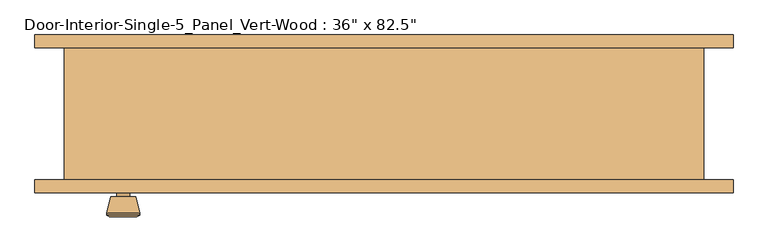
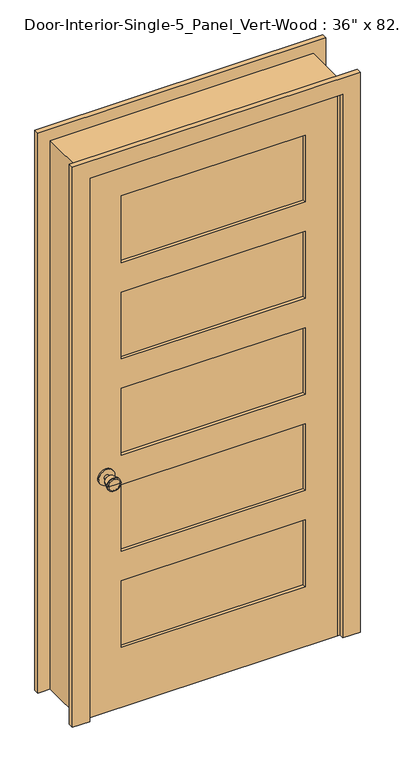
"""IFC4 building model written with IfcOpenShell, lengths in millimetres: door geometry."""

from ifc_helpers import new_model, si_unit, point, frame, frame_2d, origin, place, context, project, spatial, polyline, circle_curve, trimmed, segment, composite_curve, outline, extrude, faceted_brep, source, transform, mapped, element, save
from ifc_brep_helpers import plane_surface, cylinder_surface, revolved_surface, advanced_brep


def door_bc447172(model_context):
    return source(origin(), model_context, "Body", "SolidModel", [
        advanced_brep(
        [(-393.7, -55.9, 914.4), (-403.7, -55.9, 914.4), (-383.7, -55.9, 914.4), (-373.2241324, -6.9, 914.4), (-414.1758676, -6.9, 914.4), (-393.7, -6.9, 914.4), (-368.7, -8.7278681, 914.4), (-418.7, -8.7278681, 914.4), (-368.7, -12.1915463, 914.4), (-418.7, -12.1915463, 914.4), (-375.063764, -36.9, 914.4), (-412.336236, -36.9, 914.4), (-383.7, -36.9, 914.4), (-403.7, -36.9, 914.4)],
        [
            (0, 1),
            (1, 2, circle_curve(frame((-393.7, -55.9, 914.4), z_axis=(0.0, -1.0, 0.0), x_axis=(-1.0, 0.0, 0.0)), 10.0)),
            (2, 0),
            (2, 1, circle_curve(frame((-393.7, -55.9, 914.4), z_axis=(0.0, -1.0, 0.0), x_axis=(-1.0, 0.0, 0.0)), 10.0)),
            (3, 4, circle_curve(frame((-393.7, -6.9, 914.4), z_axis=(0.0, 1.0, 0.0), x_axis=(-1.0, 0.0, 0.0)), 20.4758676)),
            (4, 5),
            (5, 3),
            (4, 3, circle_curve(frame((-393.7, -6.9, 914.4), z_axis=(0.0, 1.0, 0.0), x_axis=(-1.0, 0.0, 0.0)), 20.4758676)),
            (6, 7, circle_curve(frame((-393.7, -8.7278681, 914.4), z_axis=(0.0, 1.0, 0.0), x_axis=(-1.0, 0.0, 0.0)), 25.0)),
            (7, 4),
            (3, 6),
            (7, 6, circle_curve(frame((-393.7, -8.7278681, 914.4), z_axis=(0.0, 1.0, 0.0), x_axis=(-1.0, 0.0, 0.0)), 25.0)),
            (8, 9, circle_curve(frame((-393.7, -12.1915463, 914.4), z_axis=(0.0, 1.0, 0.0), x_axis=(-1.0, 0.0, 0.0)), 25.0)),
            (9, 7),
            (6, 8),
            (9, 8, circle_curve(frame((-393.7, -12.1915463, 914.4), z_axis=(0.0, 1.0, 0.0), x_axis=(-1.0, 0.0, 0.0)), 25.0)),
            (10, 11, circle_curve(frame((-393.7, -36.9, 914.4), z_axis=(0.0, 1.0, 0.0), x_axis=(-1.0, 0.0, 0.0)), 18.636236)),
            (11, 9),
            (8, 10),
            (11, 10, circle_curve(frame((-393.7, -36.9, 914.4), z_axis=(0.0, 1.0, 0.0), x_axis=(-1.0, 0.0, 0.0)), 18.636236)),
            (12, 13, circle_curve(frame((-393.7, -36.9, 914.4), z_axis=(0.0, 1.0, 0.0), x_axis=(-1.0, 0.0, 0.0)), 10.0)),
            (13, 11),
            (10, 12),
            (13, 12, circle_curve(frame((-393.7, -36.9, 914.4), z_axis=(0.0, 1.0, 0.0), x_axis=(-1.0, 0.0, 0.0)), 10.0)),
            (1, 13),
            (12, 2),
        ],
        [
            plane_surface(frame((-393.7, -55.9, 914.4), z_axis=(0.0, -1.0, 0.0), x_axis=(-1.0, 0.0, 0.0))),
            plane_surface(frame((-393.7, -6.9, 914.4), z_axis=(0.0, 1.0, 0.0), x_axis=(-1.0, 0.0, 0.0))),
            revolved_surface(polyline([(-414.1758676, -6.9, 914.4), (-418.7, -8.7278681, 914.4)]), (-393.7, -55.9, 914.4), (0.0, -1.0, 0.0)),
            cylinder_surface(frame((-393.7, -55.9, 914.4), z_axis=(0.0, -1.0, 0.0), x_axis=(-1.0, 0.0, 0.0)), 25.0),
            revolved_surface(polyline([(-418.7, -12.1915463, 914.4), (-412.336236, -36.9, 914.4)]), (-393.7, -55.9, 914.4), (0.0, -1.0, 0.0)),
            plane_surface(frame((-393.7, -36.9, 914.4), z_axis=(0.0, -1.0, 0.0), x_axis=(-1.0, 0.0, 0.0))),
            cylinder_surface(frame((-393.7, -55.9, 914.4), z_axis=(0.0, -1.0, 0.0), x_axis=(-1.0, 0.0, 0.0)), 10.0),
        ],
        [
            (0, [[1, 2, 3]]),
            (0, [[-3, 4, -1]]),
            (1, [[5, 6, 7]]),
            (1, [[8, -7, -6]]),
            (2, [[9, 10, -5, 11]]),
            (2, [[12, -11, -8, -10]]),
            (3, [[13, 14, -9, 15]]),
            (3, [[16, -15, -12, -14]]),
            (4, [[17, 18, -13, 19]]),
            (4, [[20, -19, -16, -18]]),
            (5, [[21, 22, -17, 23]]),
            (5, [[24, -23, -20, -22]]),
            (6, [[-2, 25, -21, 26]]),
            (6, [[-4, -26, -24, -25]]),
        ],
    ),
        extrude(outline(composite_curve([segment(trimmed(circle_curve(frame_2d((914.4, -393.7)), 30.0), [point((914.4, -423.7))], [point((914.4, -363.7))], False, "CARTESIAN"), True, "CONTINUOUS"), segment(trimmed(circle_curve(frame_2d((914.4, -393.7)), 30.0), [point((914.4, -363.7))], [point((914.4, -423.7))], False, "CARTESIAN"), True, "CONTINUOUS")], self_intersect=False)), frame((0.0, -61.9, 0.0), z_axis=(0.0, 1.0, 0.0), x_axis=(0.0, 0.0, 1.0)), (0.0, 0.0, 1.0), 6.0),
        advanced_brep(
        [(-393.7, -102.825, 914.4), (-383.7, -102.825, 914.4), (-403.7, -102.825, 914.4), (-373.2241324, -151.825, 914.4), (-393.7, -151.825, 914.4), (-414.1758676, -151.825, 914.4), (-368.7, -149.9971319, 914.4), (-418.7, -149.9971319, 914.4), (-368.7, -146.5334537, 914.4), (-418.7, -146.5334537, 914.4), (-375.063764, -121.825, 914.4), (-412.336236, -121.825, 914.4), (-383.7, -121.825, 914.4), (-403.7, -121.825, 914.4)],
        [
            (0, 1),
            (1, 2, circle_curve(frame((-393.7, -102.825, 914.4), z_axis=(0.0, 1.0, 0.0), x_axis=(-1.0, 0.0, 0.0)), 10.0)),
            (2, 0),
            (2, 1, circle_curve(frame((-393.7, -102.825, 914.4), z_axis=(0.0, 1.0, 0.0), x_axis=(-1.0, 0.0, 0.0)), 10.0)),
            (3, 4),
            (4, 5),
            (5, 3, circle_curve(frame((-393.7, -151.825, 914.4), z_axis=(0.0, -1.0, 0.0), x_axis=(-1.0, 0.0, 0.0)), 20.4758676)),
            (3, 5, circle_curve(frame((-393.7, -151.825, 914.4), z_axis=(0.0, -1.0, 0.0), x_axis=(-1.0, 0.0, 0.0)), 20.4758676)),
            (6, 3),
            (5, 7),
            (7, 6, circle_curve(frame((-393.7, -149.9971319, 914.4), z_axis=(0.0, -1.0, 0.0), x_axis=(-1.0, 0.0, 0.0)), 25.0)),
            (6, 7, circle_curve(frame((-393.7, -149.9971319, 914.4), z_axis=(0.0, -1.0, 0.0), x_axis=(-1.0, 0.0, 0.0)), 25.0)),
            (8, 6),
            (7, 9),
            (9, 8, circle_curve(frame((-393.7, -146.5334537, 914.4), z_axis=(0.0, -1.0, 0.0), x_axis=(-1.0, 0.0, 0.0)), 25.0)),
            (8, 9, circle_curve(frame((-393.7, -146.5334537, 914.4), z_axis=(0.0, -1.0, 0.0), x_axis=(-1.0, 0.0, 0.0)), 25.0)),
            (10, 8),
            (9, 11),
            (11, 10, circle_curve(frame((-393.7, -121.825, 914.4), z_axis=(0.0, -1.0, 0.0), x_axis=(-1.0, 0.0, 0.0)), 18.636236)),
            (10, 11, circle_curve(frame((-393.7, -121.825, 914.4), z_axis=(0.0, -1.0, 0.0), x_axis=(-1.0, 0.0, 0.0)), 18.636236)),
            (12, 10),
            (11, 13),
            (13, 12, circle_curve(frame((-393.7, -121.825, 914.4), z_axis=(0.0, -1.0, 0.0), x_axis=(-1.0, 0.0, 0.0)), 10.0)),
            (12, 13, circle_curve(frame((-393.7, -121.825, 914.4), z_axis=(0.0, -1.0, 0.0), x_axis=(-1.0, 0.0, 0.0)), 10.0)),
            (1, 12),
            (13, 2),
        ],
        [
            plane_surface(frame((-393.7, -102.825, 914.4), z_axis=(0.0, 1.0, 0.0), x_axis=(-1.0, 0.0, 0.0))),
            plane_surface(frame((-393.7, -151.825, 914.4), z_axis=(0.0, -1.0, 0.0), x_axis=(-1.0, 0.0, 0.0))),
            revolved_surface(polyline([(-414.1758676, -151.825, 914.4), (-418.7, -149.9971319, 914.4)]), (-393.7, -102.825, 914.4), (0.0, 1.0, 0.0)),
            cylinder_surface(frame((-393.7, -102.825, 914.4), z_axis=(0.0, 1.0, 0.0), x_axis=(-1.0, 0.0, 0.0)), 25.0),
            revolved_surface(polyline([(-418.7, -146.5334537, 914.4), (-412.336236, -121.825, 914.4)]), (-393.7, -102.825, 914.4), (0.0, 1.0, 0.0)),
            plane_surface(frame((-393.7, -121.825, 914.4), z_axis=(0.0, 1.0, 0.0), x_axis=(-1.0, 0.0, 0.0))),
            cylinder_surface(frame((-393.7, -102.825, 914.4), z_axis=(0.0, 1.0, 0.0), x_axis=(-1.0, 0.0, 0.0)), 10.0),
        ],
        [
            (0, [[1, 2, 3]]),
            (0, [[-3, 4, -1]]),
            (1, [[5, 6, 7]]),
            (1, [[-6, -5, 8]]),
            (2, [[9, -7, 10, 11]]),
            (2, [[-10, -8, -9, 12]]),
            (3, [[13, -11, 14, 15]]),
            (3, [[-14, -12, -13, 16]]),
            (4, [[17, -15, 18, 19]]),
            (4, [[-18, -16, -17, 20]]),
            (5, [[21, -19, 22, 23]]),
            (5, [[-22, -20, -21, 24]]),
            (6, [[25, -23, 26, -2]]),
            (6, [[-26, -24, -25, -4]]),
        ],
    ),
        extrude(outline(composite_curve([segment(trimmed(circle_curve(frame_2d((914.4, -393.7)), 30.0), [point((914.4, -423.7))], [point((914.4, -363.7))], False, "CARTESIAN"), True, "CONTINUOUS"), segment(trimmed(circle_curve(frame_2d((914.4, -393.7)), 30.0), [point((914.4, -363.7))], [point((914.4, -423.7))], False, "CARTESIAN"), True, "CONTINUOUS")], self_intersect=False)), frame((0.0, -102.825, 0.0), z_axis=(0.0, 1.0, 0.0), x_axis=(0.0, 0.0, 1.0)), (0.0, 0.0, 1.0), 6.0),
        faceted_brep([(482.6, -96.825, 0.0), (457.2, -96.825, 0.0), (457.2, -61.9, 0.0), (444.5, -61.9, 0.0), (444.5, -26.975, 0.0), (457.2, -26.975, 0.0), (457.2, 103.175, 0.0), (482.6, 103.175, 0.0), (482.6, 103.175, 2125.4), (482.6, -96.825, 2125.4), (457.2, 103.175, 2100.0), (-457.2, 103.175, 2100.0), (-457.2, 103.175, 0.0), (-482.6, 103.175, 0.0), (-482.6, 103.175, 2125.4), (457.2, -26.975, 2100.0), (444.5, -26.975, 2087.3), (-444.5, -26.975, 2087.3), (-444.5, -26.975, 0.0), (-457.2, -26.975, 0.0), (-457.2, -26.975, 2100.0), (444.5, -61.9, 2087.3), (457.2, -61.9, 2100.0), (-457.2, -61.9, 2100.0), (-457.2, -61.9, 0.0), (-444.5, -61.9, 0.0), (-444.5, -61.9, 2087.3), (457.2, -96.825, 2100.0), (-482.6, -96.825, 2125.4), (-482.6, -96.825, 0.0), (-457.2, -96.825, 0.0), (-457.2, -96.825, 2100.0)], [[[0, 1, 2, 3, 4, 5, 6, 7]], [[7, 8, 9, 0]], [[6, 10, 11, 12, 13, 14, 8, 7]], [[5, 15, 10, 6]], [[4, 16, 17, 18, 19, 20, 15, 5]], [[3, 21, 16, 4]], [[2, 22, 23, 24, 25, 26, 21, 3]], [[1, 27, 22, 2]], [[0, 9, 28, 29, 30, 31, 27, 1]], [[8, 14, 28, 9]], [[15, 20, 11, 10]], [[21, 26, 17, 16]], [[27, 31, 23, 22]], [[29, 13, 12, 19, 18, 25, 24, 30]], [[14, 13, 29, 28]], [[20, 19, 12, 11]], [[26, 25, 18, 17]], [[31, 30, 24, 23]]]),
        extrude(outline(polyline([(2100.0, -457.2), (0.0, -457.2), (0.0, 457.2), (2100.0, 457.2), (2100.0, -457.2)]), holes=[polyline([(1980.9375, -336.55), (1980.9375, 336.55), (1722.545, 336.55), (1722.545, -336.55), (1980.9375, -336.55)]), polyline([(490.1675, -336.55), (490.1675, 336.55), (231.775, 336.55), (231.775, -336.55), (490.1675, -336.55)]), polyline([(1235.5525, -336.55), (1235.5525, 336.55), (977.16, 336.55), (977.16, -336.55), (1235.5525, -336.55)]), polyline([(1608.245, -336.55), (1608.245, 336.55), (1349.8525, 336.55), (1349.8525, -336.55), (1608.245, -336.55)]), polyline([(862.86, -336.55), (862.86, 336.55), (604.4675, 336.55), (604.4675, -336.55), (862.86, -336.55)])]), frame((0.0, -96.825, 0.0), z_axis=(0.0, 1.0, 0.0), x_axis=(0.0, 0.0, 1.0)), (0.0, 0.0, 1.0), 34.925),
        extrude(outline(polyline([(336.55, -73.5416667), (336.55, -85.1833333), (-336.55, -85.1833333), (-336.55, -73.5416667), (336.55, -73.5416667)])), frame((0.0, 0.0, 1722.545), z_axis=(0.0, 0.0, 1.0), x_axis=(1.0, 0.0, 0.0)), (0.0, 0.0, 1.0), 258.3925),
        extrude(outline(polyline([(336.55, -73.5416667), (336.55, -85.1833333), (-336.55, -85.1833333), (-336.55, -73.5416667), (336.55, -73.5416667)])), frame((0.0, 0.0, 1349.8525), z_axis=(0.0, 0.0, 1.0), x_axis=(1.0, 0.0, 0.0)), (0.0, 0.0, 1.0), 258.3925),
        extrude(outline(polyline([(336.55, -73.5416667), (336.55, -85.1833333), (-336.55, -85.1833333), (-336.55, -73.5416667), (336.55, -73.5416667)])), frame((0.0, 0.0, 604.4675), z_axis=(0.0, 0.0, 1.0), x_axis=(1.0, 0.0, 0.0)), (0.0, 0.0, 1.0), 258.3925),
        extrude(outline(polyline([(336.55, -73.5416667), (336.55, -85.1833333), (-336.55, -85.1833333), (-336.55, -73.5416667), (336.55, -73.5416667)])), frame((0.0, 0.0, 231.775), z_axis=(0.0, 0.0, 1.0), x_axis=(1.0, 0.0, 0.0)), (0.0, 0.0, 1.0), 258.3925),
        extrude(outline(polyline([(336.55, -73.5416667), (336.55, -85.1833333), (-336.55, -85.1833333), (-336.55, -73.5416667), (336.55, -73.5416667)])), frame((0.0, 0.0, 977.16), z_axis=(0.0, 0.0, 1.0), x_axis=(1.0, 0.0, 0.0)), (0.0, 0.0, 1.0), 258.3925),
        extrude(outline(polyline([(0.0, 527.05), (2169.85, 527.05), (2169.85, -527.05), (0.0, -527.05), (0.0, -463.55), (2106.35, -463.55), (2106.35, 463.55), (0.0, 463.55), (0.0, 527.05)])), frame((0.0, -115.875, 0.0), z_axis=(0.0, 1.0, 0.0), x_axis=(0.0, 0.0, 1.0)), (0.0, 0.0, 1.0), 19.05),
        extrude(outline(polyline([(0.0, 527.05), (2169.85, 527.05), (2169.85, -527.05), (0.0, -527.05), (0.0, -463.55), (2106.35, -463.55), (2106.35, 463.55), (0.0, 463.55), (0.0, 527.05)])), frame((0.0, 103.175, 0.0), z_axis=(0.0, 1.0, 0.0), x_axis=(0.0, 0.0, 1.0)), (0.0, 0.0, 1.0), 19.05),
    ])


if __name__ == "__main__":
    model = new_model("IFC4")
    model_context = context("Model", 3, world=origin())
    ifc_project = project(units=[si_unit("LENGTHUNIT", "METRE", prefix="MILLI")], contexts=[model_context])
    site = spatial("IfcSite", under=ifc_project)
    building = spatial("IfcBuilding", under=site)
    placement = place(None, origin())
    door_shape = door_bc447172(model_context)
    element("IfcDoor", 1, ObjectType="Door-Interior-Single-5_Panel_Vert-Wood : 36\" x 82.5\"", at=placement, inside=building, context=model_context, shape_type="MappedRepresentation", body=[
        mapped(door_shape, transform((0.0, 0.0, 0.0), x_axis=(1.0, 0.0, 0.0), y_axis=(0.0, 1.0, 0.0), z_axis=(0.0, 0.0, 1.0))),
    ])
    save(model, "model.ifc")

# Revit data of these elements
# Type "Door-Interior-Single-5_Panel_Vert-Wood : 36\" x 82.5\""
#   Type Mark = "20"
#   Assembly Code = "C1020300"
#   Analytic Construction = "Wooden"
#   Top Rail = 0' - 4 11/16"
#   Thickness = 0' - 1 3/8"
#   Thermal Resistance (R) = 2.5876 (h·ft²·°F)/BTU
#   Swing Angle [instance default] = 90.00°
#   Stiles = 0' - 4 3/4"
#   Rough Width = 3' - 2"
#   Rough Height = 6' - 11.67717"
#   Intermediate Rail = 0' - 4 1/2"
#   Height = 6' - 10.67717"
#   Width = 3' - 0"
#   Heat Transfer Coefficient (U) = 0.3865 BTU/(h·ft²·°F)
#   Bottom Rail = 0' - 9 1/8"
#   Trim Material = Cherry
#   Panel Material = Cherry
#   Frame Material = Cherry
#   Door Handle Material = Aluminum
#   Visual Light Transmittance = 0
#   Solar Heat Gain Coefficient = 0
#   Wall Closure = (empty or 0)
#   Function = (empty or 0)
# Element 1 (IfcDoor, "Door-Interior-Single-5_Panel_Vert-Wood : 36\" x 82.5\"")
#   Materials on its faces: "Cherry", "Aluminum"
# Materials
#   "Cherry": class "Wood", colour RGB 226 177 128, transparency 0, Description = "Prunus Serotina", Cost = 0
#   "Aluminum": class "Metal", colour RGB 247 247 247, transparency 0, Description = "Aluminum 6061", Cost = 0
